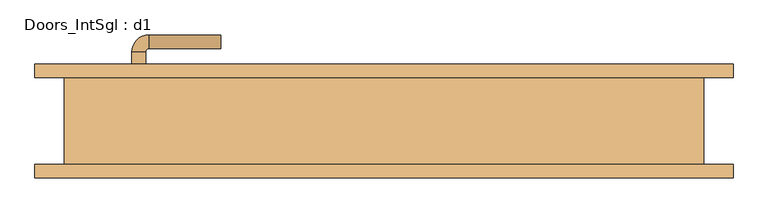
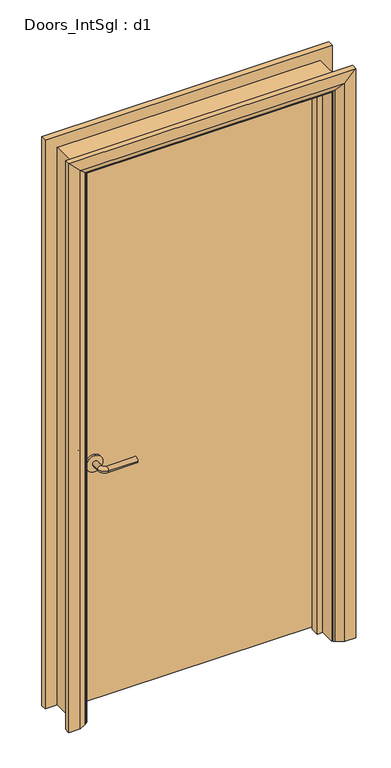
"""IFC4 building model written with IfcOpenShell, lengths in millimetres: door geometry, Doors_IntSgl : d1."""

from ifc_helpers import new_model, si_unit, point, frame, frame_2d, origin, place, context, project, spatial, polyline, circle_curve, ellipse_curve, trimmed, segment, composite_curve, outline, extrude, faceted_brep, source, transform, mapped, element, save
from ifc_brep_helpers import plane_surface, cylinder_surface, revolved_surface, advanced_brep


def doors_intsgl_d1_afe1ebc3(model_context):
    return source(origin(), model_context, "Body", "SolidModel", [
        advanced_brep(
        [(-369.25, 17.5, 900.0), (-349.25, 17.5, 900.0), (-349.25, -12.5, 900.0), (-369.25, -12.5, 900.0), (-344.25, -17.5, 900.0), (-344.25, -37.5, 900.0), (-239.25, -37.5, 900.0), (-239.25, -17.5, 900.0)],
        [
            (0, 1, circle_curve(frame((-359.25, 17.5, 900.0), z_axis=(0.0, 1.0, 0.0), x_axis=(1.0, 0.0, 0.0)), 10.0)),
            (1, 0, circle_curve(frame((-359.25, 17.5, 900.0), z_axis=(0.0, 1.0, 0.0), x_axis=(1.0, 0.0, 0.0)), 10.0)),
            (1, 2),
            (2, 3, circle_curve(frame((-359.25, -12.5, 900.0), z_axis=(0.0, 1.0, 0.0), x_axis=(1.0, 0.0, 0.0)), 10.0)),
            (3, 0),
            (3, 2, circle_curve(frame((-359.25, -12.5, 900.0), z_axis=(0.0, 1.0, 0.0), x_axis=(1.0, 0.0, 0.0)), 10.0)),
            (4, 5, circle_curve(frame((-344.25, -27.5, 900.0), z_axis=(-1.0, 0.0, 0.0), x_axis=(0.0, 1.0, 0.0)), 10.0)),
            (5, 3, circle_curve(frame((-344.25, -12.5, 900.0), z_axis=(0.0, 0.0, -1.0), x_axis=(-1.0, 0.0, 0.0)), 25.0)),
            (2, 4, circle_curve(frame((-344.25, -12.5, 900.0), z_axis=(0.0, 0.0, 1.0), x_axis=(-1.0, 0.0, 0.0)), 5.0)),
            (5, 4, circle_curve(frame((-344.25, -27.5, 900.0), z_axis=(-1.0, 0.0, 0.0), x_axis=(0.0, 1.0, 0.0)), 10.0)),
            (6, 7, circle_curve(frame((-239.25, -27.5, 900.0), z_axis=(1.0, 0.0, 0.0), x_axis=(0.0, 1.0, 0.0)), 10.0)),
            (7, 6, circle_curve(frame((-239.25, -27.5, 900.0), z_axis=(1.0, 0.0, 0.0), x_axis=(0.0, 1.0, 0.0)), 10.0)),
            (4, 7),
            (6, 5),
        ],
        [
            plane_surface(frame((-359.25, 17.5, 900.0), z_axis=(0.0, 1.0, 0.0), x_axis=(0.0, 0.0, 1.0))),
            cylinder_surface(frame((-359.25, 17.5, 900.0), z_axis=(0.0, 1.0, 0.0), x_axis=(1.0, 0.0, 0.0)), 10.0),
            revolved_surface(trimmed(ellipse_curve(frame((-359.25, -12.5, 900.0), z_axis=(0.0, -1.0, 0.0), x_axis=(1.0, 0.0, 0.0)), 10.0, 10.0), [point((-369.25, -12.5, 900.0))], [point((-349.25, -12.5, 900.0))], True, "CARTESIAN"), (-344.25, -12.5, 900.0), (0.0, 0.0, -1.0)),
            revolved_surface(trimmed(ellipse_curve(frame((-359.25, -12.5, 900.0), z_axis=(0.0, -1.0, 0.0), x_axis=(1.0, 0.0, 0.0)), 10.0, 10.0), [point((-349.25, -12.5, 900.0))], [point((-369.25, -12.5, 900.0))], True, "CARTESIAN"), (-344.25, -12.5, 900.0), (0.0, 0.0, -1.0)),
            plane_surface(frame((-239.25, -27.5, 900.0), z_axis=(1.0, 0.0, 0.0), x_axis=(0.0, 0.0, 1.0))),
            cylinder_surface(frame((-344.25, -27.5, 900.0), z_axis=(-1.0, 0.0, 0.0), x_axis=(0.0, 1.0, 0.0)), 10.0),
        ],
        [
            (0, [[1, 2]]),
            (1, [[3, 4, 5, -2]]),
            (1, [[-5, 6, -3, -1]]),
            (2, [[7, 8, -4, 9]]),
            (3, [[10, -9, -6, -8]]),
            (4, [[11, 12]]),
            (5, [[13, -11, 14, -7]]),
            (5, [[-14, -12, -13, -10]]),
        ],
    ),
        extrude(outline(composite_curve([segment(trimmed(circle_curve(frame_2d((900.0, -361.75)), 30.0), [point((900.0, -391.75))], [point((900.0, -331.75))], False, "CARTESIAN"), True, "CONTINUOUS"), segment(trimmed(circle_curve(frame_2d((900.0, -361.75)), 30.0), [point((900.0, -331.75))], [point((900.0, -391.75))], False, "CARTESIAN"), True, "CONTINUOUS")], self_intersect=False)), frame((0.0, 17.5, 0.0), z_axis=(0.0, 1.0, 0.0), x_axis=(0.0, 0.0, 1.0)), (0.0, 0.0, 1.0), 8.0),
        advanced_brep(
        [(-369.25, 71.5, 900.0), (-349.25, 71.5, 900.0), (-369.25, 101.5, 900.0), (-349.25, 101.5, 900.0), (-344.25, 106.5, 900.0), (-344.25, 126.5, 900.0), (-239.25, 126.5, 900.0), (-239.25, 106.5, 900.0)],
        [
            (0, 1, circle_curve(frame((-359.25, 71.5, 900.0), z_axis=(0.0, -1.0, 0.0), x_axis=(1.0, 0.0, 0.0)), 10.0)),
            (1, 0, circle_curve(frame((-359.25, 71.5, 900.0), z_axis=(0.0, -1.0, 0.0), x_axis=(1.0, 0.0, 0.0)), 10.0)),
            (0, 2),
            (2, 3, circle_curve(frame((-359.25, 101.5, 900.0), z_axis=(0.0, -1.0, 0.0), x_axis=(1.0, 0.0, 0.0)), 10.0)),
            (3, 1),
            (3, 2, circle_curve(frame((-359.25, 101.5, 900.0), z_axis=(0.0, -1.0, 0.0), x_axis=(1.0, 0.0, 0.0)), 10.0)),
            (4, 3, circle_curve(frame((-344.25, 101.5, 900.0), z_axis=(0.0, 0.0, 1.0), x_axis=(-1.0, 0.0, 0.0)), 5.0)),
            (2, 5, circle_curve(frame((-344.25, 101.5, 900.0), z_axis=(0.0, 0.0, -1.0), x_axis=(-1.0, 0.0, 0.0)), 25.0)),
            (5, 4, circle_curve(frame((-344.25, 116.5, 900.0), z_axis=(-1.0, 0.0, 0.0), x_axis=(0.0, -1.0, 0.0)), 10.0)),
            (4, 5, circle_curve(frame((-344.25, 116.5, 900.0), z_axis=(-1.0, 0.0, 0.0), x_axis=(0.0, -1.0, 0.0)), 10.0)),
            (6, 7, circle_curve(frame((-239.25, 116.5, 900.0), z_axis=(1.0, 0.0, 0.0), x_axis=(0.0, -1.0, 0.0)), 10.0)),
            (7, 6, circle_curve(frame((-239.25, 116.5, 900.0), z_axis=(1.0, 0.0, 0.0), x_axis=(0.0, -1.0, 0.0)), 10.0)),
            (5, 6),
            (7, 4),
        ],
        [
            plane_surface(frame((-359.25, 71.5, 900.0), z_axis=(0.0, -1.0, 0.0), x_axis=(0.0, 0.0, 1.0))),
            cylinder_surface(frame((-359.25, 71.5, 900.0), z_axis=(0.0, -1.0, 0.0), x_axis=(1.0, 0.0, 0.0)), 10.0),
            revolved_surface(trimmed(ellipse_curve(frame((-359.25, 101.5, 900.0), z_axis=(0.0, -1.0, 0.0), x_axis=(1.0, 0.0, 0.0)), 10.0, 10.0), [point((-369.25, 101.5, 900.0))], [point((-349.25, 101.5, 900.0))], True, "CARTESIAN"), (-344.25, 101.5, 900.0), (0.0, 0.0, -1.0)),
            revolved_surface(trimmed(ellipse_curve(frame((-359.25, 101.5, 900.0), z_axis=(0.0, -1.0, 0.0), x_axis=(1.0, 0.0, 0.0)), 10.0, 10.0), [point((-349.25, 101.5, 900.0))], [point((-369.25, 101.5, 900.0))], True, "CARTESIAN"), (-344.25, 101.5, 900.0), (0.0, 0.0, -1.0)),
            plane_surface(frame((-239.25, 116.5, 900.0), z_axis=(1.0, 0.0, 0.0), x_axis=(0.0, 0.0, 1.0))),
            cylinder_surface(frame((-344.25, 116.5, 900.0), z_axis=(-1.0, 0.0, 0.0), x_axis=(0.0, -1.0, 0.0)), 10.0),
        ],
        [
            (0, [[1, 2]]),
            (1, [[-1, 3, 4, 5]]),
            (1, [[-2, -5, 6, -3]]),
            (2, [[7, -4, 8, 9]]),
            (3, [[-8, -6, -7, 10]]),
            (4, [[11, 12]]),
            (5, [[-9, 13, -12, 14]]),
            (5, [[-10, -14, -11, -13]]),
        ],
    ),
        extrude(outline(composite_curve([segment(trimmed(circle_curve(frame_2d((900.0, -361.75)), 30.0), [point((900.0, -391.75))], [point((900.0, -331.75))], False, "CARTESIAN"), True, "CONTINUOUS"), segment(trimmed(circle_curve(frame_2d((900.0, -361.75)), 30.0), [point((900.0, -331.75))], [point((900.0, -391.75))], False, "CARTESIAN"), True, "CONTINUOUS")], self_intersect=False)), frame((0.0, 63.5, 0.0), z_axis=(0.0, 1.0, 0.0), x_axis=(0.0, 0.0, 1.0)), (0.0, 0.0, 1.0), 8.0),
        extrude(outline(polyline([(434.25, 25.5), (-434.25, 25.5), (-434.25, 63.5), (434.25, 63.5), (434.25, 25.5)])), frame((0.0, 0.0, 8.0), z_axis=(0.0, 0.0, 1.0), x_axis=(1.0, 0.0, 0.0)), (0.0, 0.0, 1.0), 2060.0),
        advanced_brep(
        [(511.25, 83.5, 0.0), (511.25, 63.5, 0.0), (441.25, 63.5, 0.0), (445.25, 69.5, 0.0), (471.25, 83.5, 0.0), (511.25, 83.5, 2145.0), (511.25, 63.5, 2145.0), (-511.25, 63.5, 2145.0), (-511.25, 63.5, 0.0), (-441.25, 63.5, 0.0), (-441.25, 63.5, 2075.0), (441.25, 63.5, 2075.0), (445.25, 69.5, 2079.0), (471.25, 83.5, 2105.0), (-471.25, 83.5, 2105.0), (-471.25, 83.5, 0.0), (-511.25, 83.5, 0.0), (-511.25, 83.5, 2145.0), (-445.25, 69.5, 0.0), (-445.25, 69.5, 2079.0)],
        [
            (0, 1),
            (1, 2),
            (2, 3, circle_curve(frame((449.25, 62.5, 0.0), z_axis=(0.0, 0.0, -1.0), x_axis=(1.0, 0.0, 0.0)), 8.0622577)),
            (3, 4),
            (4, 0),
            (0, 5),
            (5, 6),
            (6, 1),
            (6, 7),
            (7, 8),
            (8, 9),
            (9, 10),
            (10, 11),
            (11, 2),
            (11, 12, ellipse_curve(frame((449.25, 62.5, 2083.0), z_axis=(0.7071067811865475, 0.0, -0.7071067811865475), x_axis=(-0.7071067811865474, 0.0, -0.7071067811865476)), 11.4017543, 8.0622577)),
            (12, 3),
            (12, 13),
            (13, 4),
            (13, 14),
            (14, 15),
            (15, 16),
            (16, 17),
            (17, 5),
            (7, 17),
            (16, 8),
            (15, 18),
            (18, 9, circle_curve(frame((-449.25, 62.5, 0.0), z_axis=(0.0, 0.0, -1.0), x_axis=(-1.0, 0.0, 0.0)), 8.0622577)),
            (19, 10, ellipse_curve(frame((-449.25, 62.5, 2083.0), z_axis=(-0.7071067811865475, 0.0, -0.7071067811865475), x_axis=(-0.7071067811865474, 0.0, 0.7071067811865476)), 11.4017543, 8.0622577)),
            (18, 19),
            (14, 19),
            (19, 12),
        ],
        [
            plane_surface(frame((441.25, 63.5, 0.0), z_axis=(0.0, 0.0, -1.0), x_axis=(0.0, -1.0, 0.0))),
            plane_surface(frame((511.25, 83.5, 0.0), z_axis=(1.0, 0.0, 0.0), x_axis=(0.0, 0.0, 1.0))),
            plane_surface(frame((511.25, 63.5, 0.0), z_axis=(0.0, -1.0, 0.0), x_axis=(0.0, 0.0, 1.0))),
            cylinder_surface(frame((449.25, 62.5, 0.0), z_axis=(0.0, 0.0, -1.0), x_axis=(1.0, 0.0, 0.0)), 8.0622577),
            plane_surface(frame((445.25, 69.5, 0.0), z_axis=(-0.4740998230350126, 0.880471099922178, 0.0), x_axis=(0.0, 0.0, 1.0))),
            plane_surface(frame((471.25, 83.5, 0.0), z_axis=(0.0, 1.0, 0.0), x_axis=(0.0, 0.0, 1.0))),
            plane_surface(frame((-511.25, 83.5, 2145.0), z_axis=(-1.0, 0.0, 0.0), x_axis=(0.0, 0.0, -1.0))),
            plane_surface(frame((-441.25, 63.5, 0.0), z_axis=(0.0, 0.0, -1.0), x_axis=(0.0, -1.0, 0.0))),
            cylinder_surface(frame((-449.25, 62.5, 2075.0), z_axis=(0.0, 0.0, 1.0), x_axis=(-1.0, 0.0, 0.0)), 8.0622577),
            plane_surface(frame((-445.25, 69.5, 2079.0), z_axis=(0.47409982303501824, 0.8804710999221749, 0.0), x_axis=(0.0, 0.0, -1.0))),
            plane_surface(frame((511.25, 83.5, 2145.0), z_axis=(0.0, 0.0, 1.0), x_axis=(-1.0, 0.0, 0.0))),
            cylinder_surface(frame((441.25, 62.5, 2083.0), z_axis=(1.0, 0.0, 0.0), x_axis=(0.0, 0.0, 1.0)), 8.0622577),
            plane_surface(frame((445.25, 69.5, 2079.0), z_axis=(0.0, 0.8804710999221764, -0.4740998230350154), x_axis=(-1.0, 0.0, 0.0))),
        ],
        [
            (0, [[1, 2, 3, 4, 5]]),
            (1, [[-1, 6, 7, 8]]),
            (2, [[-2, -8, 9, 10, 11, 12, 13, 14]]),
            (3, [[-3, -14, 15, 16]]),
            (4, [[-4, -16, 17, 18]]),
            (5, [[-5, -18, 19, 20, 21, 22, 23, -6]]),
            (6, [[24, -22, 25, -10]]),
            (7, [[-21, 26, 27, -11, -25]]),
            (8, [[28, -12, -27, 29]]),
            (9, [[30, -29, -26, -20]]),
            (10, [[-7, -23, -24, -9]]),
            (11, [[-15, -13, -28, 31]]),
            (12, [[-17, -31, -30, -19]]),
        ],
    ),
        extrude(outline(polyline([(0.0, -436.25), (0.0, -417.25), (2051.0, -417.25), (2051.0, 417.25), (0.0, 417.25), (0.0, 436.25), (2070.0, 436.25), (2070.0, -436.25), (0.0, -436.25)])), frame((0.0, -8.5, 0.0), z_axis=(0.0, 1.0, 0.0), x_axis=(0.0, 0.0, 1.0)), (0.0, 0.0, 1.0), 32.0),
        advanced_brep(
        [(-511.25, -83.5, 0.0), (-511.25, -63.5, 0.0), (-441.25, -63.5, 0.0), (-445.25, -69.5, 0.0), (-471.25, -83.5, 0.0), (-511.25, -83.5, 2145.0), (-511.25, -63.5, 2145.0), (-441.25, -63.5, 2075.0), (-445.25, -69.5, 2079.0), (-471.25, -83.5, 2105.0), (511.25, -83.5, 0.0), (471.25, -83.5, 0.0), (445.25, -69.5, 0.0), (441.25, -63.5, 0.0), (511.25, -63.5, 0.0), (511.25, -83.5, 2145.0), (471.25, -83.5, 2105.0), (445.25, -69.5, 2079.0), (441.25, -63.5, 2075.0), (511.25, -63.5, 2145.0)],
        [
            (0, 1),
            (1, 2),
            (2, 3, circle_curve(frame((-449.25, -62.5, 0.0), z_axis=(0.0, 0.0, -1.0), x_axis=(-1.0, 0.0, 0.0)), 8.0622577)),
            (3, 4),
            (4, 0),
            (0, 5),
            (5, 6),
            (6, 1),
            (6, 7),
            (7, 2),
            (7, 8, ellipse_curve(frame((-449.25, -62.5, 2083.0), z_axis=(-0.7071067811865475, 0.0, -0.7071067811865475), x_axis=(0.7071067811865474, 0.0, -0.7071067811865476)), 11.4017543, 8.0622577)),
            (8, 3),
            (8, 9),
            (9, 4),
            (9, 5),
            (10, 11),
            (11, 12),
            (12, 13, circle_curve(frame((449.25, -62.5, 0.0), z_axis=(0.0, 0.0, -1.0), x_axis=(1.0, 0.0, 0.0)), 8.0622577)),
            (13, 14),
            (14, 10),
            (15, 16),
            (16, 11),
            (10, 15),
            (16, 17),
            (17, 12),
            (17, 18, ellipse_curve(frame((449.25, -62.5, 2083.0), z_axis=(0.7071067811865475, 0.0, -0.7071067811865475), x_axis=(0.7071067811865474, 0.0, 0.7071067811865476)), 11.4017543, 8.0622577)),
            (18, 13),
            (18, 19),
            (19, 14),
            (19, 15),
            (5, 15),
            (19, 6),
            (18, 7),
            (17, 8),
            (16, 9),
        ],
        [
            plane_surface(frame((-441.25, -136.3010989, 0.0), z_axis=(0.0, 0.0, -1.0), x_axis=(1.0, 0.0, 0.0))),
            plane_surface(frame((-511.25, -83.5, 0.0), z_axis=(-1.0, 0.0, 0.0), x_axis=(0.0, 0.0, 1.0))),
            plane_surface(frame((-511.25, -63.5, 0.0), z_axis=(0.0, 1.0, 0.0), x_axis=(0.0, 0.0, 1.0))),
            cylinder_surface(frame((-449.25, -62.5, 0.0), z_axis=(0.0, 0.0, -1.0), x_axis=(-1.0, 0.0, 0.0)), 8.0622577),
            plane_surface(frame((-445.25, -69.5, 0.0), z_axis=(0.4740998230350183, -0.8804710999221749, 0.0), x_axis=(0.0, 0.0, 1.0))),
            plane_surface(frame((-471.25, -83.5, 0.0), z_axis=(0.0, -1.0, 0.0), x_axis=(0.0, 0.0, 1.0))),
            plane_surface(frame((441.25, -136.3010989, 0.0), z_axis=(0.0, 0.0, -1.0), x_axis=(-1.0, 0.0, 0.0))),
            plane_surface(frame((471.25, -83.5, 2105.0), z_axis=(0.0, -1.0, 0.0), x_axis=(0.0, 0.0, -1.0))),
            plane_surface(frame((445.25, -69.5, 2079.0), z_axis=(-0.4740998230350183, -0.8804710999221749, 0.0), x_axis=(0.0, 0.0, -1.0))),
            cylinder_surface(frame((449.25, -62.5, 2075.0), z_axis=(0.0, 0.0, 1.0), x_axis=(1.0, 0.0, 0.0)), 8.0622577),
            plane_surface(frame((511.25, -63.5, 2145.0), z_axis=(0.0, 1.0, 0.0), x_axis=(0.0, 0.0, -1.0))),
            plane_surface(frame((511.25, -83.5, 2145.0), z_axis=(1.0, 0.0, 0.0), x_axis=(0.0, 0.0, -1.0))),
            plane_surface(frame((-511.25, -83.5, 2145.0), z_axis=(0.0, 0.0, 1.0), x_axis=(1.0, 0.0, 0.0))),
            plane_surface(frame((-511.25, -63.5, 2145.0), z_axis=(0.0, 1.0, 0.0), x_axis=(1.0, 0.0, 0.0))),
            cylinder_surface(frame((-441.25, -62.5, 2083.0), z_axis=(-1.0, 0.0, 0.0), x_axis=(0.0, 0.0, 1.0)), 8.0622577),
            plane_surface(frame((-445.25, -69.5, 2079.0), z_axis=(0.0, -0.8804710999221749, -0.4740998230350183), x_axis=(1.0, 0.0, 0.0))),
            plane_surface(frame((-471.25, -83.5, 2105.0), z_axis=(0.0, -1.0, 0.0), x_axis=(1.0, 0.0, 0.0))),
        ],
        [
            (0, [[1, 2, 3, 4, 5]]),
            (1, [[-1, 6, 7, 8]]),
            (2, [[-2, -8, 9, 10]]),
            (3, [[-3, -10, 11, 12]]),
            (4, [[-4, -12, 13, 14]]),
            (5, [[-5, -14, 15, -6]]),
            (6, [[16, 17, 18, 19, 20]]),
            (7, [[21, 22, -16, 23]]),
            (8, [[24, 25, -17, -22]]),
            (9, [[26, 27, -18, -25]]),
            (10, [[28, 29, -19, -27]]),
            (11, [[30, -23, -20, -29]]),
            (12, [[-7, 31, -30, 32]]),
            (13, [[-9, -32, -28, 33]]),
            (14, [[-11, -33, -26, 34]]),
            (15, [[-13, -34, -24, 35]]),
            (16, [[-15, -35, -21, -31]]),
        ],
    ),
        faceted_brep([(-436.25, 63.5, 0.0), (-436.25, -63.5, 0.0), (-468.25, -63.5, 0.0), (-468.25, 63.5, 0.0), (-436.25, 63.5, 2070.0), (-436.25, -63.5, 2070.0), (-468.25, -63.5, 2102.0), (-468.25, 63.5, 2102.0), (436.25, 63.5, 0.0), (468.25, 63.5, 0.0), (468.25, -63.5, 0.0), (436.25, -63.5, 0.0), (436.25, 63.5, 2070.0), (468.25, 63.5, 2102.0), (468.25, -63.5, 2102.0), (436.25, -63.5, 2070.0)], [[[0, 1, 2, 3]], [[1, 0, 4, 5]], [[2, 1, 5, 6]], [[3, 2, 6, 7]], [[0, 3, 7, 4]], [[8, 9, 10, 11]], [[12, 13, 9, 8]], [[13, 14, 10, 9]], [[14, 15, 11, 10]], [[15, 12, 8, 11]], [[5, 4, 12, 15]], [[6, 5, 15, 14]], [[7, 6, 14, 13]], [[4, 7, 13, 12]]]),
    ])


if __name__ == "__main__":
    model = new_model("IFC4")
    model_context = context("Model", 3, world=origin())
    ifc_project = project(units=[si_unit("LENGTHUNIT", "METRE", prefix="MILLI")], contexts=[model_context])
    site = spatial("IfcSite", under=ifc_project)
    building = spatial("IfcBuilding", under=site)
    placement = place(None, origin())
    doors_intsgl_d1_shape = doors_intsgl_d1_afe1ebc3(model_context)
    element("IfcDoor", 1, ObjectType="Doors_IntSgl : d1", at=placement, inside=building, context=model_context, shape_type="MappedRepresentation", body=[
        mapped(doors_intsgl_d1_shape, transform((0.0, 0.0, 0.0), x_axis=(1.0, 0.0, 0.0), y_axis=(0.0, 1.0, 0.0), z_axis=(0.0, 0.0, 1.0))),
    ])
    save(model, "model.ifc")

# Revit data of these elements
# Type "Doors_IntSgl : d1"
#   Type Mark = "46"
#   Type Comments = "Internal Single"
#   Operation = "SingleSwingRight"
#   Manufacturer = "Revit"
#   Keynote = "L20"
#   Description = "Internal Single Door"
#   Analytic Construction = "Metal"
#   UnderCut = 0' - 0.31496"
#   Tolerance = 0' - 0.07874"
#   Thickness = 0' - 1.49606"
#   Thermal Resistance (R) = 0.270117 (m²·K)/W
#   Structural Tolerance = 0' - 0.31496"
#   StopDepth = 0' - 1.25984"
#   Stop Thickness = 0' - 0.74803"
#   Rough Width = 3' - 1 1/2"
#   Rough Height = 6' - 11.07087"
#   Height to Top Lock Rail = 3' - 3.37008"
#   Heat Transfer Coefficient (U) = 3.7021 W/(m²·K)
#   Handle Z Distance = 2' - 11.43307"
#   Handle X Distance = 0' - 2.95276"
#   Frame Thickness = 0' - 1.25984"
#   Door Panel Width = 2' - 10.19291"
#   Door Panel Thickness = 0' - 1.49606"
#   Door Panel Offset = 0' - 0"
#   Height = 6' - 11.07087"
#   Width = 3' - 1 1/2"
#   Door Panel Height = 6' - 9.10236"
#   Architrave Setback = 0' - 0.19685"
#   Vis - Ironmongery = yes
#   Material Ironmongery = Door - Handle
#   Material Frame = Door - Frame/Mullion (1)
#   Material Door = Door - Panel
#   Material Architrave = Door - Architrave
#   Visual Light Transmittance = 0
#   Solar Heat Gain Coefficient = 0
#   Function = (empty or 0)
#   Wall Closure = (empty or 0)
# Element 1 (IfcDoor, "Doors_IntSgl : d1")
#   Materials on its faces: "Door - Architrave", "Door - Handle", "Door - Frame/Mullion (1)", "Door - Panel"
# Materials
#   "Door - Handle": colour RGB 0 0 0, transparency 0, Keynote = "P21", Cost = 0
#   "Door - Frame/Mullion (1)": class "Wood", colour RGB 212 179 113, transparency 0, Keynote = "L20", Cost = 0
#   "Door - Panel": class "Wood", colour RGB 210 159 95, transparency 0, Keynote = "L20", Cost = 0
#   "Door - Architrave": class "Wood", colour RGB 154 90 5, transparency 0, Keynote = "P20", Cost = 0
